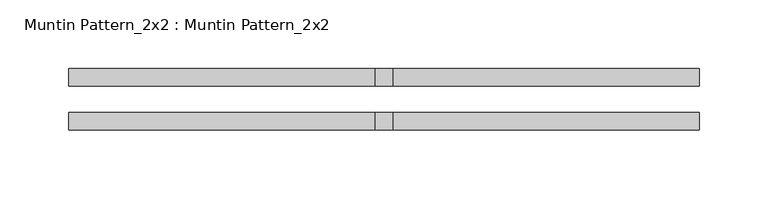
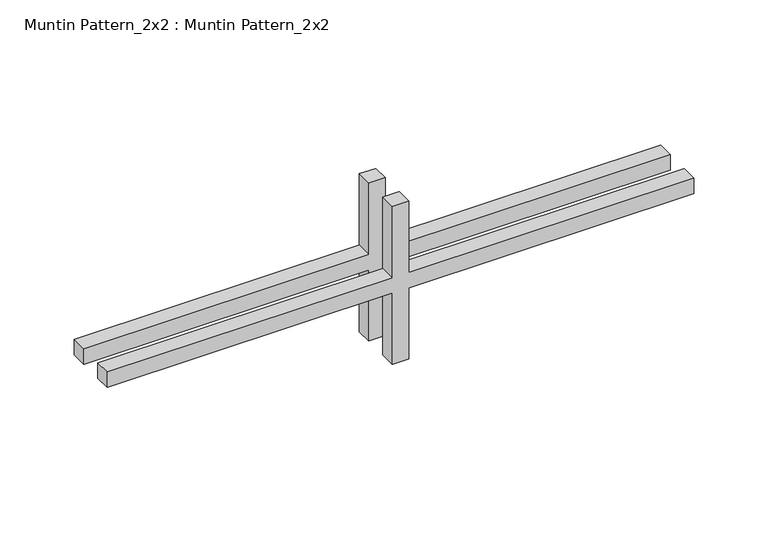
"""IFC4 building model written with IfcOpenShell, lengths in millimetres: proxy geometry, Muntin Pattern_2x2 : Muntin Pattern_2x2."""

from ifc_helpers import new_model, si_unit, frame, origin, place, context, project, spatial, polyline, outline, extrude, source, transform, mapped, element, save


def muntin_pattern_2x2_muntin_pattern_2x2_019d64ce(model_context):
    return source(origin(), model_context, "Body", "SweptSolid", [
        extrude(outline(polyline([(71.4375, -6.35), (71.4375, -228.6), (58.7375, -228.6), (58.7375, -6.35), (0.0, -6.35), (0.0, 6.35), (58.7375, 6.35), (58.7375, 228.6), (71.4375, 228.6), (71.4375, 6.35), (130.175, 6.35), (130.175, -6.35), (71.4375, -6.35)])), frame((0.0, 9.525, 0.0), z_axis=(0.0, 1.0, 0.0), x_axis=(0.0, 0.0, 1.0)), (0.0, 0.0, 1.0), 12.7),
        extrude(outline(polyline([(71.4375, -6.35), (71.4375, -228.6), (58.7375, -228.6), (58.7375, -6.35), (0.0, -6.35), (0.0, 6.35), (58.7375, 6.35), (58.7375, 228.6), (71.4375, 228.6), (71.4375, 6.35), (130.175, 6.35), (130.175, -6.35), (71.4375, -6.35)])), frame((0.0, -22.225, 0.0), z_axis=(0.0, 1.0, 0.0), x_axis=(0.0, 0.0, 1.0)), (0.0, 0.0, 1.0), 12.7),
    ])


if __name__ == "__main__":
    model = new_model("IFC4")
    model_context = context("Model", 3, world=origin())
    ifc_project = project(units=[si_unit("LENGTHUNIT", "METRE", prefix="MILLI")], contexts=[model_context])
    site = spatial("IfcSite", under=ifc_project)
    building = spatial("IfcBuilding", under=site)
    placement = place(None, origin())
    muntin_pattern_2x2_muntin_pattern_2x2_shape = muntin_pattern_2x2_muntin_pattern_2x2_019d64ce(model_context)
    element("IfcBuildingElementProxy", 1, Name="Muntin Pattern_2x2 : Muntin Pattern_2x2", ObjectType="Muntin Pattern_2x2 : Muntin Pattern_2x2", at=placement, inside=building, context=model_context, shape_type="MappedRepresentation", body=[
        mapped(muntin_pattern_2x2_muntin_pattern_2x2_shape, transform((0.0, 0.0, 0.0), x_axis=(1.0, 0.0, 0.0), y_axis=(0.0, 1.0, 0.0), z_axis=(0.0, 0.0, 1.0))),
    ])
    save(model, "model.ifc")

# Revit data of these elements
# Type "Muntin Pattern_2x2 : Muntin Pattern_2x2"
#   Width [instance default] = 4' - 0"
#   Thickness = 0' - 0 1/2"
#   Height [instance default] = 4' - 0"
#   Distance = 0' - 0 3/4"
#   Interior Material [instance default] = none
#   Exterior Material [instance default] = none
#   Default Elevation = 0
# Element 1 (IfcBuildingElementProxy, "Muntin Pattern_2x2 : Muntin Pattern_2x2")
#   Width = 1' - 6"
#   Height = 0' - 5 1/8"
#   Interior Material = Wood - Stained
#   Exterior Material = Clad - White
#   Materials on its faces: "Clad - White", "Wood - Stained"
# Materials
#   "Clad - White": class "Wood", colour RGB 242 242 238, transparency 0, Cost = 0
#   "Wood - Stained": class "Wood", colour RGB 224 178 126, transparency 0, Cost = 0
